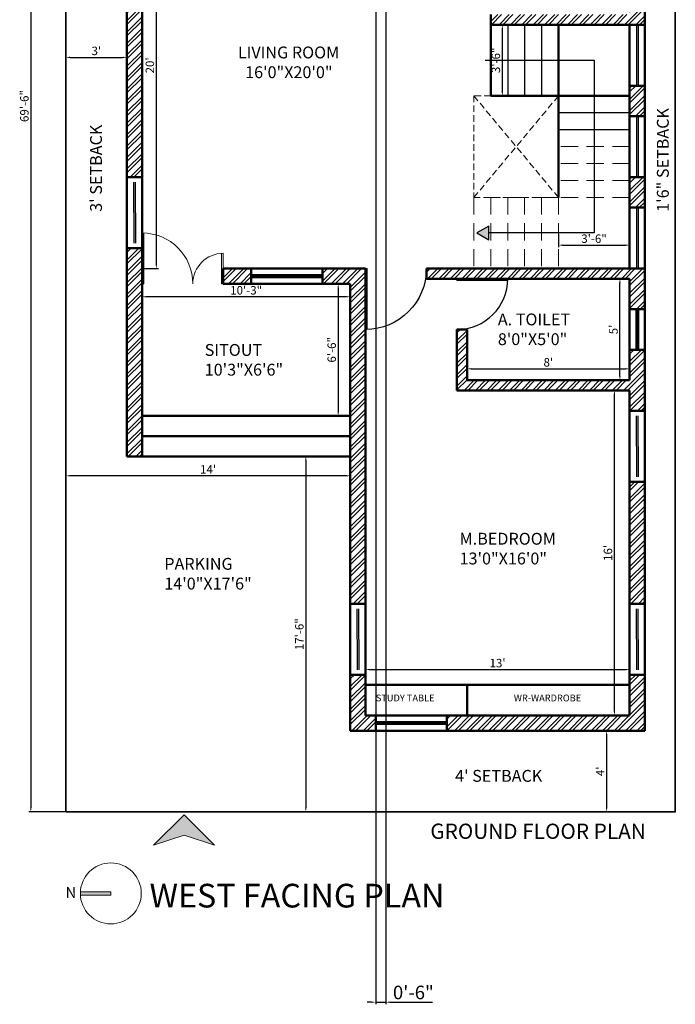
# Model space of a CAD drawing. Units: inches. Extents: x 1986 to 21484, y -1816 to 2016.
# Tile 81 of 85: x 4810 to 5197, y 953 to 1535. Entities that reach past the tile are written whole.
import ezdxf

# ---------------------------------------------------------------- set-up
doc = ezdxf.new("R2010")
doc.units = ezdxf.units.IN
doc.linetypes.add('DASHED', pattern=[19.05, 12.7, -6.35])
for name, color, linetype, lineweight in [('A-ANNO-DIMS', 2, 'Continuous', 18), ('A-ANNO-SYMB', 1, 'Continuous', 18), ('A-ANNO-TEXT', 7, 'Continuous', 18), ('A-AREA-IDEN', 3, 'Continuous', 18), ('A-DOOR', 3, 'Continuous', 25), ('A-FLOR-STRS', 7, 'Continuous', 25), ('A-FLOR-STRS-OVHD', 8, 'DASHED', 18), ('A-FURN', 8, 'Continuous', 18), ('A-GLAZ', 4, 'Continuous', 25), ('A-WALL', 7, 'Continuous', 50), ('A-WALL-PATT', 8, 'Continuous', 13), ('C-PROP', 7, 'Continuous', 35)]:
    doc.layers.add(name, color=color, linetype=linetype, lineweight=lineweight)
doc.styles.get("Standard").update_dxf_attribs({"font": 'arial.ttf'})
doc.dimstyles.new('ISO-25', dxfattribs={"dimtxt": 8, "dimasz": 2.5, "dimexe": 1.25, "dimexo": 0.625, "dimtad": 1, "dimdec": 1, "dimlunit": 3, "dimtxsty": 'Standard', "dimcen": 2.5, "dimadec": 0, "dimazin": 0, "dimtfac": 1, "dimtdec": 1, "dimtmove": 0, "dimatfit": 3, "dimfxl": 1, "dimarcsym": 0})

# ---------------------------------------------------------------- blocks, each defined once
blk = doc.blocks.new('MD')
for p, q in [((1902.58, 1512.86), (1902.58, 1482.86)), ((1903.58, 1512.86), (1903.58, 1482.86)), ((1949.58, 1482.86), (1949.58, 1500.86)), ((1950.58, 1482.86), (1950.58, 1500.86)), ((1902.58, 1482.86), (1903.58, 1482.86)), ((1949.58, 1482.86), (1950.58, 1482.86))]:
    blk.add_line(p, q)
for centre, radius, start, end in [((1902.58, 1482.86), 30, 0, 90), ((1950.58, 1482.86), 18, 90, 180)]:
    blk.add_arc(centre, radius, start, end)
blk = doc.blocks.new('D2')
for p, q in [((1722.5, 1505.46), (1722.5, 1475.46)), ((1723.5, 1505.46), (1723.5, 1475.46)), ((1722.5, 1475.46), (1723.5, 1475.46))]:
    blk.add_line(p, q)
blk.add_arc((1722.5, 1475.46), 30, 0, 90)
blk = doc.blocks.new('D1')
for p, q in [((1805.96, 1500.36), (1805.96, 1464.36)), ((1806.96, 1500.36), (1806.96, 1464.36)), ((1805.96, 1464.36), (1806.96, 1464.36))]:
    blk.add_line(p, q)
blk.add_arc((1805.96, 1464.36), 36, 0, 90)
blk = doc.blocks.new('*D42')
at = {"layer": 'A-ANNO-DIMS', "color": 0, "lineweight": -2, "transparency": 16777216}
for p, q in [((4882.51, 1627.75), (4891.58, 1627.75)), ((4890.33, 1390.25), (4890.33, 1625.25)), ((4882.51, 1387.75), (4891.58, 1387.75))]:
    blk.add_line(p, q, dxfattribs=at)
at = {"layer": 'A-ANNO-DIMS', "color": 0, "transparency": 16777216}
for points in [[(4889.91, 1625.25), (4890.74, 1625.25), (4890.33, 1627.75)], [(4889.91, 1390.25), (4890.74, 1390.25), (4890.33, 1387.75)]]:
    blk.add_solid(points, dxfattribs=at)
at = {"layer": 'Defpoints', "color": 0, "transparency": 16777216}
for p in [(4881.89, 1627.75), (4890.33, 1627.75), (4881.89, 1387.75)]:
    blk.add_point(p, dxfattribs=at)
at = {"layer": 'A-ANNO-DIMS', "color": 0, "transparency": 16777216, "insert": (4887.15, 1507.75), "char_height": 5, "attachment_point": 5, "rotation": 90}
blk.add_mtext("20'", dxfattribs=at)
blk = doc.blocks.new('*D45')
at = {"layer": 'A-ANNO-DIMS', "color": 0, "lineweight": -2, "transparency": 16777216}
for p, q in [((5093.46, 1531.75), (5095.95, 1531.75)), ((5094.7, 1529.25), (5094.7, 1492.25)), ((5093.46, 1489.75), (5095.95, 1489.75))]:
    blk.add_line(p, q, dxfattribs=at)
at = {"layer": 'A-ANNO-DIMS', "color": 0, "transparency": 16777216}
for points in [[(5094.28, 1529.25), (5095.12, 1529.25), (5094.7, 1531.75)], [(5094.28, 1492.25), (5095.12, 1492.25), (5094.7, 1489.75)]]:
    blk.add_solid(points, dxfattribs=at)
at = {"layer": 'Defpoints', "color": 0, "transparency": 16777216}
for p in [(5092.84, 1531.75), (5092.84, 1489.75), (5094.7, 1489.75)]:
    blk.add_point(p, dxfattribs=at)
at = {"layer": 'A-ANNO-DIMS', "color": 0, "transparency": 16777216, "insert": (5091.52, 1510.75), "char_height": 5, "attachment_point": 5, "rotation": 90}
blk.add_mtext('3\'-6"', dxfattribs=at)
blk = doc.blocks.new('*D46')
at = {"layer": 'A-ANNO-DIMS', "color": 0, "lineweight": -2, "transparency": 16777216}
for p, q in [((5127.89, 1408.13), (5127.89, 1400.31)), ((5169.89, 1408.13), (5169.89, 1400.31)), ((5130.39, 1401.56), (5167.39, 1401.56))]:
    blk.add_line(p, q, dxfattribs=at)
at = {"layer": 'A-ANNO-DIMS', "color": 0, "transparency": 16777216}
for points in [[(5130.39, 1401.98), (5130.39, 1401.14), (5127.89, 1401.56)], [(5167.39, 1401.98), (5167.39, 1401.14), (5169.89, 1401.56)]]:
    blk.add_solid(points, dxfattribs=at)
at = {"layer": 'Defpoints', "color": 0, "transparency": 16777216}
for p in [(5127.89, 1408.75), (5169.89, 1408.75), (5169.89, 1401.56)]:
    blk.add_point(p, dxfattribs=at)
at = {"layer": 'A-ANNO-DIMS', "color": 0, "transparency": 16777216, "insert": (5148.89, 1404.74), "char_height": 5, "attachment_point": 5}
blk.add_mtext('3\'-6"', dxfattribs=at)
blk = doc.blocks.new('*D47')
at = {"layer": 'A-ANNO-DIMS', "color": 0, "lineweight": -2, "transparency": 16777216}
for p, q in [((5073.89, 1322.38), (5073.89, 1329.76)), ((5076.39, 1328.51), (5167.39, 1328.51)), ((5169.89, 1322.38), (5169.89, 1329.76))]:
    blk.add_line(p, q, dxfattribs=at)
at = {"layer": 'A-ANNO-DIMS', "color": 0, "transparency": 16777216}
for points in [[(5076.39, 1328.93), (5076.39, 1328.1), (5073.89, 1328.51)], [(5167.39, 1328.93), (5167.39, 1328.1), (5169.89, 1328.51)]]:
    blk.add_solid(points, dxfattribs=at)
at = {"layer": 'Defpoints', "color": 0, "transparency": 16777216}
for p in [(5169.89, 1328.51), (5073.89, 1321.75), (5169.89, 1321.75)]:
    blk.add_point(p, dxfattribs=at)
at = {"layer": 'A-ANNO-DIMS', "color": 0, "transparency": 16777216, "insert": (5121.89, 1331.69), "char_height": 5, "attachment_point": 5}
blk.add_mtext("8'", dxfattribs=at)
blk = doc.blocks.new('*D48')
at = {"layer": 'A-ANNO-DIMS', "color": 0, "lineweight": -2, "transparency": 16777216}
for p, q in [((5169.26, 1381.75), (5162.92, 1381.75)), ((5164.17, 1324.25), (5164.17, 1379.25)), ((5169.26, 1321.75), (5162.92, 1321.75))]:
    blk.add_line(p, q, dxfattribs=at)
at = {"layer": 'A-ANNO-DIMS', "color": 0, "transparency": 16777216}
for points in [[(5163.75, 1379.25), (5164.59, 1379.25), (5164.17, 1381.75)], [(5163.75, 1324.25), (5164.59, 1324.25), (5164.17, 1321.75)]]:
    blk.add_solid(points, dxfattribs=at)
at = {"layer": 'Defpoints', "color": 0, "transparency": 16777216}
for p in [(5164.17, 1381.75), (5169.89, 1381.75), (5169.89, 1321.75)]:
    blk.add_point(p, dxfattribs=at)
at = {"layer": 'A-ANNO-DIMS', "color": 0, "transparency": 16777216, "insert": (5161, 1351.75), "char_height": 5, "attachment_point": 5, "rotation": 90}
blk.add_mtext("5'", dxfattribs=at)
blk = doc.blocks.new('*D49')
at = {"layer": 'A-ANNO-DIMS', "color": 0, "lineweight": -2, "transparency": 16777216}
for p, q in [((5004.26, 1378.75), (4996.49, 1378.75)), ((4997.74, 1376.25), (4997.74, 1303.25)), ((5004.26, 1300.75), (4996.49, 1300.75))]:
    blk.add_line(p, q, dxfattribs=at)
at = {"layer": 'A-ANNO-DIMS', "color": 0, "transparency": 16777216}
for points in [[(4997.33, 1376.25), (4998.16, 1376.25), (4997.74, 1378.75)], [(4997.33, 1303.25), (4998.16, 1303.25), (4997.74, 1300.75)]]:
    blk.add_solid(points, dxfattribs=at)
at = {"layer": 'Defpoints', "color": 0, "transparency": 16777216}
for p in [(5004.89, 1378.75), (4997.74, 1300.75), (5004.89, 1300.75)]:
    blk.add_point(p, dxfattribs=at)
at = {"layer": 'A-ANNO-DIMS', "color": 0, "transparency": 16777216, "insert": (4994.57, 1339.75), "char_height": 5, "attachment_point": 5, "rotation": 90}
blk.add_mtext('6\'-6"', dxfattribs=at)
blk = doc.blocks.new('*D50')
at = {"layer": 'A-ANNO-DIMS', "color": 0, "lineweight": -2, "transparency": 16777216}
for p, q in [((4881.89, 1378.13), (4881.89, 1369.82)), ((5004.89, 1378.13), (5004.89, 1369.82)), ((5002.39, 1371.07), (4884.39, 1371.07))]:
    blk.add_line(p, q, dxfattribs=at)
at = {"layer": 'A-ANNO-DIMS', "color": 0, "transparency": 16777216}
for points in [[(4884.39, 1371.49), (4884.39, 1370.66), (4881.89, 1371.07)], [(5002.39, 1371.49), (5002.39, 1370.66), (5004.89, 1371.07)]]:
    blk.add_solid(points, dxfattribs=at)
at = {"layer": 'Defpoints', "color": 0, "transparency": 16777216}
for p in [(4881.89, 1378.75), (5004.89, 1378.75), (4881.89, 1371.07)]:
    blk.add_point(p, dxfattribs=at)
at = {"layer": 'A-ANNO-DIMS', "color": 0, "transparency": 16777216, "insert": (4943.39, 1374.25), "char_height": 5, "attachment_point": 5}
blk.add_mtext('10\'-3"', dxfattribs=at)
blk = doc.blocks.new('*D51')
at = {"layer": 'A-ANNO-DIMS', "color": 0, "lineweight": -2, "transparency": 16777216}
for p, q in [((5013.89, 1142.38), (5013.89, 1152.08)), ((5169.89, 1142.38), (5169.89, 1152.08)), ((5016.39, 1150.83), (5167.39, 1150.83))]:
    blk.add_line(p, q, dxfattribs=at)
at = {"layer": 'A-ANNO-DIMS', "color": 0, "transparency": 16777216}
for points in [[(5016.39, 1151.25), (5016.39, 1150.41), (5013.89, 1150.83)], [(5167.39, 1151.25), (5167.39, 1150.41), (5169.89, 1150.83)]]:
    blk.add_solid(points, dxfattribs=at)
at = {"layer": 'Defpoints', "color": 0, "transparency": 16777216}
for p in [(5169.89, 1150.83), (5013.89, 1141.75), (5169.89, 1141.75)]:
    blk.add_point(p, dxfattribs=at)
at = {"layer": 'A-ANNO-DIMS', "color": 0, "transparency": 16777216, "insert": (5091.89, 1154.01), "char_height": 5, "attachment_point": 5}
blk.add_mtext("13'", dxfattribs=at)
blk = doc.blocks.new('*D52')
at = {"layer": 'A-ANNO-DIMS', "color": 0, "lineweight": -2, "transparency": 16777216}
for p, q in [((5169.26, 1315.75), (5159.69, 1315.75)), ((5160.94, 1126.25), (5160.94, 1313.25)), ((5169.26, 1123.75), (5159.69, 1123.75))]:
    blk.add_line(p, q, dxfattribs=at)
at = {"layer": 'A-ANNO-DIMS', "color": 0, "transparency": 16777216}
for points in [[(5160.52, 1313.25), (5161.35, 1313.25), (5160.94, 1315.75)], [(5160.52, 1126.25), (5161.35, 1126.25), (5160.94, 1123.75)]]:
    blk.add_solid(points, dxfattribs=at)
at = {"layer": 'Defpoints', "color": 0, "transparency": 16777216}
for p in [(5160.94, 1315.75), (5169.89, 1315.75), (5169.89, 1123.75)]:
    blk.add_point(p, dxfattribs=at)
at = {"layer": 'A-ANNO-DIMS', "color": 0, "transparency": 16777216, "insert": (5157.76, 1219.75), "char_height": 5, "attachment_point": 5, "rotation": 90}
blk.add_mtext("16'", dxfattribs=at)
blk = doc.blocks.new('*D75')
at = {"layer": 'A-ANNO-DIMS', "color": 0, "lineweight": -2, "transparency": 16777216}
for p, q in [((4978.63, 1274.25), (4978.63, 1069.25)), ((4979.26, 1276.75), (4979.88, 1276.75)), ((4979.26, 1066.75), (4979.88, 1066.75))]:
    blk.add_line(p, q, dxfattribs=at)
at = {"layer": 'A-ANNO-DIMS', "color": 0, "transparency": 16777216}
for points in [[(4978.22, 1274.25), (4979.05, 1274.25), (4978.63, 1276.75)], [(4978.22, 1069.25), (4979.05, 1069.25), (4978.63, 1066.75)]]:
    blk.add_solid(points, dxfattribs=at)
at = {"layer": 'Defpoints', "color": 0, "transparency": 16777216}
for p in [(4978.63, 1276.75), (4978.63, 1066.75), (4978.63, 1066.75)]:
    blk.add_point(p, dxfattribs=at)
at = {"layer": 'A-ANNO-DIMS', "color": 0, "transparency": 16777216, "insert": (4975.45, 1171.75), "char_height": 5, "attachment_point": 5, "rotation": 90}
blk.add_mtext('17\'-6"', dxfattribs=at)
blk = doc.blocks.new('*D76')
at = {"layer": 'A-ANNO-DIMS', "color": 0, "lineweight": -2, "transparency": 16777216}
for p, q in [((4836.89, 1265.95), (4836.89, 1266.57)), ((5002.39, 1265.32), (4839.39, 1265.32)), ((5004.89, 1265.95), (5004.89, 1266.57))]:
    blk.add_line(p, q, dxfattribs=at)
at = {"layer": 'A-ANNO-DIMS', "color": 0, "transparency": 16777216}
for points in [[(4839.39, 1265.74), (4839.39, 1264.91), (4836.89, 1265.32)], [(5002.39, 1265.74), (5002.39, 1264.91), (5004.89, 1265.32)]]:
    blk.add_solid(points, dxfattribs=at)
at = {"layer": 'Defpoints', "color": 0, "transparency": 16777216}
for p in [(4836.89, 1265.32), (4836.89, 1265.32), (5004.89, 1265.32)]:
    blk.add_point(p, dxfattribs=at)
at = {"layer": 'A-ANNO-DIMS', "color": 0, "transparency": 16777216, "insert": (4920.89, 1268.46), "char_height": 5, "attachment_point": 5}
blk.add_mtext("14'", dxfattribs=at)
blk = doc.blocks.new('*D77')
at = {"layer": 'A-ANNO-DIMS', "color": 0, "lineweight": -2, "transparency": 16777216}
for p, q in [((4836.89, 1513.11), (4836.89, 1513.74)), ((4839.39, 1512.49), (4870.39, 1512.49)), ((4872.89, 1513.11), (4872.89, 1513.74))]:
    blk.add_line(p, q, dxfattribs=at)
at = {"layer": 'A-ANNO-DIMS', "color": 0, "transparency": 16777216}
for points in [[(4839.39, 1512.91), (4839.39, 1512.07), (4836.89, 1512.49)], [(4870.39, 1512.91), (4870.39, 1512.07), (4872.89, 1512.49)]]:
    blk.add_solid(points, dxfattribs=at)
at = {"layer": 'Defpoints', "color": 0, "transparency": 16777216}
for p in [(4836.89, 1512.49), (4872.89, 1512.49), (4872.89, 1512.49)]:
    blk.add_point(p, dxfattribs=at)
at = {"layer": 'A-ANNO-DIMS', "color": 0, "transparency": 16777216, "insert": (4854.89, 1515.67), "char_height": 5, "attachment_point": 5}
blk.add_mtext("3'", dxfattribs=at)
blk = doc.blocks.new('*D80')
at = {"layer": 'A-ANNO-DIMS', "color": 0, "lineweight": -2, "transparency": 16777216}
for p, q in [((5156.33, 1112.25), (5156.33, 1069.25)), ((5156.95, 1114.75), (5157.58, 1114.75)), ((5156.95, 1066.75), (5157.58, 1066.75))]:
    blk.add_line(p, q, dxfattribs=at)
at = {"layer": 'A-ANNO-DIMS', "color": 0, "transparency": 16777216}
for points in [[(5155.91, 1112.25), (5156.74, 1112.25), (5156.33, 1114.75)], [(5155.91, 1069.25), (5156.74, 1069.25), (5156.33, 1066.75)]]:
    blk.add_solid(points, dxfattribs=at)
at = {"layer": 'Defpoints', "color": 0, "transparency": 16777216}
for p in [(5156.33, 1114.75), (5156.33, 1066.75), (5156.33, 1066.75)]:
    blk.add_point(p, dxfattribs=at)
at = {"layer": 'A-ANNO-DIMS', "color": 0, "transparency": 16777216, "insert": (5153.2, 1090.75), "char_height": 5, "attachment_point": 5, "rotation": 90}
blk.add_mtext("4'", dxfattribs=at)
blk = doc.blocks.new('*D81')
at = {"layer": 'A-ANNO-DIMS', "color": 0, "lineweight": -2, "transparency": 16777216}
for p, q in [((4836.26, 1900.75), (4814.95, 1900.75)), ((4816.2, 1898.25), (4816.2, 1069.25)), ((4836.26, 1066.75), (4814.95, 1066.75))]:
    blk.add_line(p, q, dxfattribs=at)
at = {"layer": 'A-ANNO-DIMS', "color": 0, "transparency": 16777216}
for points in [[(4815.78, 1898.25), (4816.61, 1898.25), (4816.2, 1900.75)], [(4815.78, 1069.25), (4816.61, 1069.25), (4816.2, 1066.75)]]:
    blk.add_solid(points, dxfattribs=at)
at = {"layer": 'Defpoints', "color": 0, "transparency": 16777216}
for p in [(4836.89, 1900.75), (4816.2, 1066.75), (4836.89, 1066.75)]:
    blk.add_point(p, dxfattribs=at)
at = {"layer": 'A-ANNO-DIMS', "color": 0, "transparency": 16777216, "insert": (4813.02, 1483.75), "char_height": 5, "attachment_point": 5, "rotation": 90}
blk.add_mtext('69\'-6"', dxfattribs=at)
blk = doc.blocks.new('WIN-36')
for p, q in [((0, 36), (0, 0)), ((0, 36), (0, 0)), ((1, 36), (1, 0))]:
    blk.add_line(p, q)
blk = doc.blocks.new('*D132')
at = {"layer": 'A-ANNO-DIMS', "color": 0, "lineweight": -2, "transparency": 16777216}
for p, q in [((5019.89, 1627.13), (5019.89, 953.11)), ((5025.89, 1627.13), (5025.89, 953.11)), ((5017.39, 954.36), (5014.89, 954.36)), ((5019.89, 954.36), (5025.89, 954.36)), ((5028.39, 954.36), (5053.4, 954.36))]:
    blk.add_line(p, q, dxfattribs=at)
at = {"layer": 'A-ANNO-DIMS', "color": 0, "transparency": 16777216}
for points in [[(5017.39, 954.78), (5017.39, 953.95), (5019.89, 954.36)], [(5028.39, 954.78), (5028.39, 953.95), (5025.89, 954.36)]]:
    blk.add_solid(points, dxfattribs=at)
at = {"layer": 'Defpoints', "color": 0, "transparency": 16777216}
for p in [(5019.89, 1627.75), (5025.89, 1627.75), (5025.89, 954.36)]:
    blk.add_point(p, dxfattribs=at)
at = {"layer": 'A-ANNO-DIMS', "color": 0, "transparency": 16777216, "insert": (5042.15, 959.07), "char_height": 8, "attachment_point": 5}
blk.add_mtext('0\'-6"', dxfattribs=at)

msp = doc.modelspace()

# ---------------------------------------------------------------- hatches: boundary and pattern name
at = {"layer": 'A-ANNO-SYMB'}
h = msp.add_hatch(color=256, dxfattribs=at)
h.dxf.hatch_style = 1
h.paths.add_polyline_path([(4906.68, 1065.1), (4888.68, 1047.1), (4906.68, 1053.1), (4924.68, 1047.1)])
h = msp.add_hatch(color=256, dxfattribs=at)
h.dxf.hatch_style = 1
h.paths.add_polyline_path([(4845.47, 1019.61, 0.013897), (4845.45, 1018.61, 0.013897), (4845.47, 1017.61), (4863.45, 1017.61), (4863.45, 1019.61)])
at = {"layer": 'A-FLOR-STRS'}
h = msp.add_hatch(color=256, dxfattribs=at)
h.dxf.hatch_style = 1
h.paths.add_polyline_path([(5079.73, 1408.75), (5086.68, 1404.74), (5086.68, 1412.77)])
at = {"layer": 'A-WALL-PATT'}
h = msp.add_hatch(dxfattribs=at)
h.set_pattern_fill('ANSI32', color=256, scale=0.5)
h.set_pattern_definition([(45, (1297.9813, 0), (-3.367596, 3.367596), []), (45, (1300.2263, 0), (-3.367596, 3.367596), [])])
h.paths.add_polyline_path([(4929.89, 1852.75), (4872.89, 1852.75), (4872.89, 1753.75), (4881.89, 1753.75), (4881.89, 1843.75), (4929.89, 1843.75)])
h.paths.add_polyline_path([(5025.89, 1852.75), (4971.89, 1852.75), (4971.89, 1843.75), (5019.89, 1843.75), (5019.89, 1627.75), (5025.89, 1627.75)])
h.paths.add_polyline_path([(5178.89, 1852.75), (5055.89, 1852.75), (5055.89, 1843.75), (5169.89, 1843.75), (5169.89, 1795.75), (5073.89, 1795.75), (5073.89, 1813.75), (5067.89, 1813.75), (5067.89, 1789.75), (5169.89, 1789.75), (5169.89, 1741.75), (5178.89, 1741.75)])
h.paths.add_polyline_path([(5178.89, 1705.75), (5169.89, 1705.75), (5169.89, 1600.75), (5178.89, 1600.75)])
h.paths.add_polyline_path([(4983.89, 1687.75), (4881.89, 1687.75), (4881.89, 1711.75), (4872.89, 1711.75), (4872.89, 1669.75), (4881.89, 1669.75), (4881.89, 1681.75), (4971.89, 1681.75), (4971.89, 1663.75), (4977.89, 1663.75), (4977.89, 1681.75), (4983.89, 1681.75)])
h.paths.add_polyline_path([(4881.89, 1399.75), (4872.89, 1399.75), (4872.89, 1276.75), (4881.89, 1276.75)])
h.paths.add_polyline_path([(4946.39, 1387.75), (4929.89, 1387.75), (4929.89, 1378.75), (4946.39, 1378.75)])
h.paths.add_polyline_path([(5013.89, 1387.75), (4988.39, 1387.75), (4988.39, 1378.75), (5004.89, 1378.75), (5004.89, 1189.75), (5013.89, 1189.75)])
h.paths.add_polyline_path([(5178.89, 1387.75), (5169.89, 1387.75), (5049.89, 1387.75), (5049.89, 1381.75), (5169.89, 1381.75), (5169.89, 1363.75), (5178.89, 1363.75)])
h.paths.add_polyline_path([(5178.89, 1441.75), (5169.89, 1441.75), (5169.89, 1423.75), (5178.89, 1423.75)])
h.paths.add_polyline_path([(5178.89, 1495.75), (5169.89, 1495.75), (5169.89, 1477.75), (5178.89, 1477.75)])
h.paths.add_polyline_path([(5178.89, 1339.75), (5169.89, 1339.75), (5169.89, 1321.75), (5073.89, 1321.75), (5073.89, 1351.75), (5067.89, 1351.75), (5067.89, 1315.75), (5169.89, 1315.75), (5169.89, 1303.75), (5178.89, 1303.75)])
h.paths.add_polyline_path([(5178.89, 1261.75), (5169.89, 1261.75), (5169.89, 1189.75), (5178.89, 1189.75)])
h.paths.add_polyline_path([(5178.89, 1147.75), (5169.89, 1147.75), (5169.89, 1123.75), (5061.89, 1123.75), (5061.89, 1114.75), (5178.89, 1114.75)])
h.paths.add_polyline_path([(5019.89, 1123.75), (5013.89, 1123.75), (5013.89, 1147.75), (5004.89, 1147.75), (5004.89, 1114.75), (5019.89, 1114.75)])
h.paths.add_polyline_path([(5178.89, 1564.75), (5169.89, 1564.75), (5169.89, 1537.75), (5087.89, 1537.75), (5087.89, 1531.75), (5169.89, 1531.75), (5178.89, 1531.75)])
h.paths.add_polyline_path([(4881.89, 1627.75), (4977.89, 1627.75), (4977.89, 1633.75), (4947.89, 1633.75), (4881.89, 1633.75), (4881.89, 1645.75), (4872.89, 1645.75), (4872.89, 1441.75), (4881.89, 1441.75)])
h.paths.add_polyline_path([(5031.24, 1736.83), (5031.24, 1685.78), (5039.78, 1685.78), (5039.78, 1736.83)], flags=9)
h.paths.add_polyline_path([(5061.79, 1864.73), (5110.75, 1864.73), (5110.75, 1891.35), (5061.79, 1891.35)], flags=9)
h.paths.add_polyline_path([(5095.95, 1806.84), (5139.77, 1806.84), (5139.77, 1833.45), (5095.95, 1833.45)], flags=25)
h.paths.add_polyline_path([(5077.23, 1690.08), (5131.36, 1690.08), (5131.36, 1716.69), (5077.23, 1716.69)], flags=9)
h.paths.add_polyline_path([(5103.21, 1565.41), (5147.01, 1565.41), (5147.01, 1592.03), (5103.21, 1592.03)], flags=9)
h.paths.add_polyline_path([(4936.55, 1496.24), (5009.24, 1496.24), (5009.24, 1522.85), (4936.55, 1522.85)], flags=9)
h.paths.add_polyline_path([(4915.95, 1320.51), (4964.91, 1320.51), (4964.91, 1347.12), (4915.95, 1347.12)], flags=9)
h.paths.add_polyline_path([(5066.5, 1208.98), (5134.5, 1208.98), (5134.5, 1235.59), (5066.5, 1235.59)], flags=9)
h.paths.add_polyline_path([(5089.68, 1338.54), (5142.51, 1338.54), (5142.51, 1365.15), (5089.68, 1365.15)], flags=9)
h.paths.add_polyline_path([(4912.83, 1758.76), (4969.06, 1758.76), (4969.06, 1785.38), (4912.83, 1785.38)], flags=9)
h.paths.add_polyline_path([(4901.36, 1642.68), (4953.09, 1642.68), (4953.09, 1669.29), (4901.36, 1669.29)], flags=9)

# ---------------------------------------------------------------- linework, layer by layer
at = {"layer": 'A-ANNO-SYMB'}
for p, q in [((4906.68, 1065.1), (4888.68, 1047.1)), ((4906.68, 1065.1), (4924.68, 1047.1)), ((4888.68, 1047.1), (4906.68, 1053.1)), ((4906.68, 1053.1), (4888.68, 1047.1)), ((4924.68, 1047.1), (4906.68, 1053.1)), ((4906.68, 1053.1), (4924.68, 1047.1)), ((4863.45, 1019.61), (4845.45, 1019.61)), ((4863.45, 1019.61), (4863.45, 1017.61)), ((4863.45, 1017.61), (4845.45, 1017.61))]:
    msp.add_line(p, q, dxfattribs=at)
msp.add_circle((4863.45, 1018.61), 18, dxfattribs=at)
at = {"layer": 'A-FLOR-STRS'}
for p, q in [((5097.89, 1531.75), (5097.89, 1489.75)), ((5107.89, 1531.75), (5107.89, 1489.75)), ((5117.89, 1531.75), (5117.89, 1489.75)), ((5169.89, 1479.75), (5127.89, 1479.75)), ((5169.89, 1469.75), (5127.89, 1469.75))]:
    msp.add_line(p, q, dxfattribs=at)
msp.add_lwpolyline([(5084.48, 1510.75), (5148.89, 1510.75), (5148.89, 1408.75), (5086.68, 1408.75)], dxfattribs=at)
msp.add_lwpolyline([(5079.73, 1408.75), (5086.68, 1404.74), (5086.68, 1412.77)], close=True, dxfattribs=at)
at = {"layer": 'A-FLOR-STRS-OVHD', "ltscale": 0.3}
for p, q in [((5077.89, 1489.75), (5127.89, 1429.75)), ((5077.89, 1429.75), (5127.89, 1489.75))]:
    msp.add_line(p, q, dxfattribs=at)
at = {"layer": 'A-FLOR-STRS-OVHD', "ltscale": 0.8}
for p, q in [((5169.89, 1459.75), (5127.89, 1459.75)), ((5169.89, 1449.75), (5127.89, 1449.75)), ((5169.89, 1439.75), (5127.89, 1439.75)), ((5077.89, 1429.75), (5077.89, 1387.75)), ((5169.89, 1429.75), (5077.89, 1429.75)), ((5087.89, 1429.75), (5087.89, 1387.75)), ((5097.89, 1429.75), (5097.89, 1387.75)), ((5107.89, 1429.75), (5107.89, 1387.75)), ((5117.89, 1429.75), (5117.89, 1387.75)), ((5127.89, 1429.75), (5127.89, 1387.75))]:
    msp.add_line(p, q, dxfattribs=at)
at = {"layer": 'A-FLOR-STRS-OVHD', "ltscale": 0.3}
msp.add_lwpolyline([(5077.89, 1429.75), (5127.89, 1429.75), (5127.89, 1489.75), (5077.89, 1489.75)], close=True, dxfattribs=at)
at = {"layer": 'A-WALL'}
for p, q in [((5178.89, 1900.75), (5178.89, 1114.75)), ((4872.89, 1276.75), (4872.89, 1852.75)), ((4881.89, 1276.75), (4881.89, 1627.75)), ((5087.89, 1537.75), (5087.89, 1489.75)), ((5087.89, 1531.75), (5169.89, 1531.75)), ((5127.89, 1531.75), (5127.89, 1429.75)), ((5169.89, 1531.75), (5169.89, 1387.75)), ((5169.89, 1531.75), (5178.89, 1531.75)), ((5169.89, 1495.75), (5178.89, 1495.75)), ((5169.89, 1489.75), (5087.89, 1489.75)), ((5169.89, 1477.75), (5178.89, 1477.75)), ((4872.89, 1441.75), (4881.89, 1441.75)), ((5169.89, 1441.75), (5178.89, 1441.75)), ((5169.89, 1423.75), (5178.89, 1423.75)), ((4872.89, 1399.75), (4881.89, 1399.75)), ((4929.89, 1378.75), (4929.89, 1387.75)), ((4929.89, 1387.75), (5013.89, 1387.75)), ((4946.39, 1378.75), (4946.39, 1387.75)), ((4988.39, 1378.75), (4988.39, 1387.75)), ((5013.89, 1123.75), (5013.89, 1387.75)), ((5049.89, 1387.75), (5169.89, 1387.75)), ((5049.89, 1381.75), (5049.89, 1387.75)), ((5169.89, 1387.75), (5178.89, 1387.75)), ((4929.89, 1378.75), (5004.89, 1378.75)), ((4946.39, 1383.75), (4988.39, 1383.75)), ((4946.39, 1382.75), (4988.39, 1382.75)), ((5004.89, 1114.75), (5004.89, 1378.75)), ((5049.89, 1381.75), (5169.89, 1381.75)), ((5169.89, 1381.75), (5169.89, 1321.75)), ((5169.89, 1363.75), (5178.89, 1363.75)), ((5173.89, 1339.75), (5173.89, 1363.75)), ((5174.89, 1339.75), (5174.89, 1363.75)), ((5067.89, 1351.75), (5067.89, 1315.75)), ((5067.89, 1351.75), (5073.89, 1351.75)), ((5073.89, 1351.75), (5073.89, 1321.75)), ((5169.89, 1339.75), (5178.89, 1339.75)), ((5073.89, 1321.75), (5169.89, 1321.75)), ((5067.89, 1315.75), (5169.89, 1315.75)), ((5169.89, 1315.75), (5169.89, 1123.75)), ((5169.89, 1303.75), (5178.89, 1303.75)), ((4881.89, 1300.75), (5004.89, 1300.75)), ((4881.89, 1288.75), (5004.89, 1288.75)), ((4872.89, 1276.75), (5004.89, 1276.75)), ((5169.89, 1261.75), (5178.89, 1261.75)), ((5004.89, 1189.75), (5013.89, 1189.75)), ((5169.89, 1189.75), (5178.89, 1189.75)), ((5004.89, 1147.75), (5013.89, 1147.75)), ((5169.89, 1147.75), (5178.89, 1147.75)), ((5013.89, 1141.75), (5169.89, 1141.75)), ((5073.89, 1123.75), (5073.89, 1141.75)), ((5013.89, 1123.75), (5169.89, 1123.75)), ((5019.89, 1114.75), (5019.89, 1123.75)), ((5061.89, 1114.75), (5061.89, 1123.75)), ((5019.89, 1119.75), (5061.89, 1119.75)), ((5019.89, 1118.75), (5061.89, 1118.75)), ((5178.89, 1114.75), (5004.89, 1114.75))]:
    msp.add_line(p, q, dxfattribs=at)
at = {"layer": 'C-PROP'}
msp.add_lwpolyline([(4836.89, 1900.75), (5196.89, 1900.75), (5196.89, 1066.75), (4836.89, 1066.75)], close=True, dxfattribs=at)

# ---------------------------------------------------------------- block references
at = {"layer": 'A-DOOR', "xscale": -1, "rotation": 180}
msp.add_blockref('D1', (3207.92, 2852.11), dxfattribs=at)
at = {"layer": 'A-DOOR', "rotation": 270}
msp.add_blockref('D2', (3592.43, 3104.25), dxfattribs=at)
at = {"layer": 'A-FURN'}
msp.add_blockref('MD', (2979.31, -104.11), dxfattribs=at)
at = {"layer": 'A-GLAZ'}
for p in [(5173.89, 1495.75), (5173.89, 1441.75), (5173.89, 1387.75)]:
    msp.add_blockref('WIN-36', p, dxfattribs=at)
for p, rotation in [((4876.98, 1402.75), 0.302793432207276), ((5173.98, 1264.75), 0.3027934322096833), ((5008.98, 1150.75), 0.3027934322096833), ((5173.98, 1150.75), 0.3027934322096833)]:
    msp.add_blockref('WIN-36', p, dxfattribs=dict(at, rotation=rotation))

# ---------------------------------------------------------------- texts
at = {"layer": 'A-ANNO-SYMB'}
msp.add_text('N ', height=6.465, dxfattribs=at).set_placement((4836.68, 1015.88))
at = {"layer": 'A-ANNO-TEXT', "char_height": 7, "attachment_point": 1, "rotation": 90}
for s, insert in [('{\\fTimes New Roman|b0|i0|c0|p18;1\'6" SETBACK}', (5186.03, 1421.26)), ("{\\fTimes New Roman|b0|i0|c0|p18;3' SETBACK}", (4851.19, 1421.26))]:
    msp.add_mtext_dynamic_manual_height_columns(s, width=105.6127, gutter_width=12.5, heights=[0], dxfattribs=dict(at, insert=insert))
at = {"layer": 'A-ANNO-TEXT', "attachment_point": 1}
for s, width, insert, char_height in [('{\\fTimes New Roman|b0|i0|c0|p18;STUDY TABLE}', 105.6127, (5019.99, 1136.07), 4), ('{\\fTimes New Roman|b0|i0|c0|p18;WR-WARDROBE}', 105.6127, (5101.5, 1136.07), 4), ("{\\fTimes New Roman|b0|i0|c0|p18;4' SETBACK}", 105.6127, (5066.83, 1091.56), 7), ('{\\fTimes New Roman|b0|i0|c0|p18;GROUND FLOOR PLAN}', 226.7688, (5052.17, 1059.84), 9), ('{\\fTimes New Roman|b0|i0|c0|p18;WEST FACING PLAN}', 226.7688, (4886.33, 1024.3), 14)]:
    msp.add_mtext_dynamic_manual_height_columns(s, width=width, gutter_width=12.5, heights=[0], dxfattribs=dict(at, insert=insert, char_height=char_height))
at = {"layer": 'A-AREA-IDEN', "char_height": 7, "attachment_point": 1}
for s, width, insert in [('{\\fTimes New Roman|b0|i0|c0|p18;LIVING ROOM\\P  16\'0"X20\'0"}', 122.2228, (4938.5, 1518.89)), ('{\\fTimes New Roman|b0|i0|c0|p18;A. TOILET\\P8\'0"X5\'0"}', 105.6127, (5092.05, 1361.19)), ('{\\fTimes New Roman|b0|i0|c0|p18;SITOUT\\P10\'3"X6\'6"}', 105.6127, (4918.91, 1343.16)), ('{\\fTimes New Roman|b0|i0|c0|p18;M.BEDROOM \\P13\'0"X16\'0"}', 105.6127, (5069.46, 1231.63)), ('{\\fTimes New Roman|b0|i0|c0|p18;PARKING\\P14\'0"X17\'6"}', 105.6127, (4895.03, 1216.8))]:
    msp.add_mtext_dynamic_manual_height_columns(s, width=width, gutter_width=12.5, heights=[0], dxfattribs=dict(at, insert=insert))

# ---------------------------------------------------------------- dimensions: what is measured, and where the dimension line sits
at = {"layer": 'A-ANNO-DIMS'}
for base, p1, p2, angle, picture, middle in [((4816.2, 1066.75), (4836.89, 1900.75), (4836.89, 1066.75), 90, '*D81', (4813.02, 1483.75)), ((4890.33, 1627.75), (4881.89, 1387.75), (4881.89, 1627.75), 90, '*D42', (4887.15, 1507.75)), ((5094.7, 1489.75), (5092.84, 1531.75), (5092.84, 1489.75), 90, '*D45', (5091.52, 1510.75)), ((4997.74, 1300.75), (5004.89, 1378.75), (5004.89, 1300.75), 90, '*D49', (4994.57, 1339.75)), ((5164.17, 1381.75), (5169.89, 1321.75), (5169.89, 1381.75), 270, '*D48', (5161, 1351.75)), ((5160.94, 1315.75), (5169.89, 1123.75), (5169.89, 1315.75), 270, '*D52', (5157.76, 1219.75)), ((4978.63, 1066.75), (4978.63, 1276.75), (4978.63, 1066.75), 90, '*D75', (4975.45, 1171.75)), ((5156.33, 1066.75), (5156.33, 1114.75), (5156.33, 1066.75), 90, '*D80', (5153.2, 1090.75))]:
    dim = msp.add_linear_dim(base=base, p1=p1, p2=p2, angle=angle, dimstyle='ISO-25', override={"dimtxt": 5, "dimclrd": 0, "dimclre": 0, "dimclrt": 0}, dxfattribs=at)
    dim.commit()
    dim.dimension.update_dxf_attribs({"geometry": picture, "text_midpoint": middle})
for base, p1, p2, override, picture, middle in [((5025.89, 954.36), (5019.89, 1627.75), (5025.89, 1627.75), {"dimdec": 1, "dimlfac": 1, "dimrnd": 0, "dimzin": 1, "dimdsep": 46, "dimlunit": 4, "dimfrac": 2}, '*D132', (5042.15, 959.07)), ((4872.89, 1512.49), (4836.89, 1512.49), (4872.89, 1512.49), {"dimtxt": 5, "dimclrd": 0, "dimclre": 0, "dimclrt": 0}, '*D77', (4854.89, 1515.67)), ((5169.89, 1401.56), (5127.89, 1408.75), (5169.89, 1408.75), {"dimtxt": 5, "dimclrd": 0, "dimclre": 0, "dimclrt": 0}, '*D46', (5148.89, 1404.74)), ((4881.89, 1371.07), (5004.89, 1378.75), (4881.89, 1378.75), {"dimtxt": 5, "dimclrd": 0, "dimclre": 0, "dimclrt": 0}, '*D50', (4943.39, 1374.25)), ((5169.89, 1328.51), (5073.89, 1321.75), (5169.89, 1321.75), {"dimtxt": 5, "dimclrd": 0, "dimclre": 0, "dimclrt": 0}, '*D47', (5121.89, 1331.69)), ((4836.89, 1265.32), (5004.89, 1265.32), (4836.89, 1265.32), {"dimtxt": 5, "dimclrd": 0, "dimclre": 0, "dimclrt": 0}, '*D76', (4920.89, 1268.46)), ((5169.89, 1150.83), (5013.89, 1141.75), (5169.89, 1141.75), {"dimtxt": 5, "dimclrd": 0, "dimclre": 0, "dimclrt": 0}, '*D51', (5091.89, 1154.01))]:
    dim = msp.add_linear_dim(base=base, p1=p1, p2=p2, dimstyle='ISO-25', override=override, dxfattribs=at)
    dim.commit()
    dim.dimension.update_dxf_attribs({"geometry": picture, "text_midpoint": middle})

doc.saveas('drawing.dxf')
